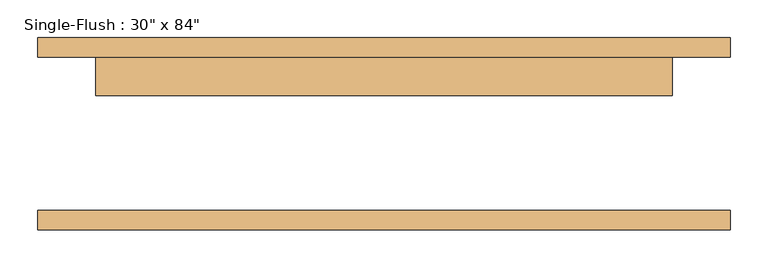
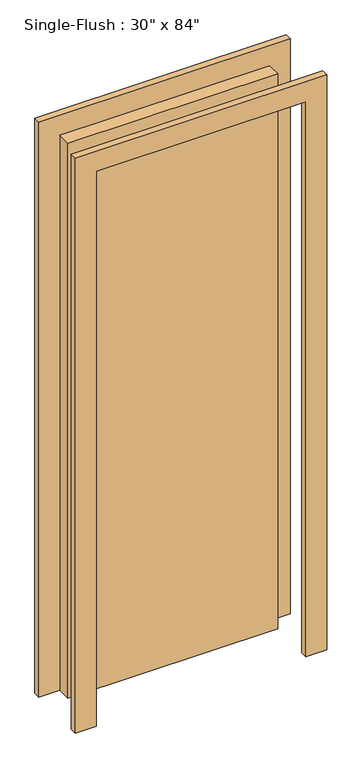
"""IFC4 building model written with IfcOpenShell, lengths in millimetres: door geometry."""

from ifc_helpers import new_model, si_unit, frame, origin, origin_with_axes, place, context, project, spatial, polyline, outline, extrude, source, transform, mapped, element, save


def door_b6acaa4e(model_context):
    return source(origin(), model_context, "Body", "SweptSolid", [
        extrude(outline(polyline([(2209.8, -457.2), (0.0, -457.2), (0.0, -381.0), (2133.6, -381.0), (2133.6, 381.0), (0.0, 381.0), (0.0, 457.2), (2209.8, 457.2), (2209.8, -457.2)])), frame((0.0, 101.6, 0.0), z_axis=(0.0, 1.0, 0.0), x_axis=(0.0, 0.0, 1.0)), (0.0, 0.0, 1.0), 25.4),
        extrude(outline(polyline([(2209.8, 457.2), (2209.8, -457.2), (0.0, -457.2), (0.0, -381.0), (2133.6, -381.0), (2133.6, 381.0), (0.0, 381.0), (0.0, 457.2), (2209.8, 457.2)])), frame((0.0, -127.0, 0.0), z_axis=(0.0, 1.0, 0.0), x_axis=(0.0, 0.0, 1.0)), (0.0, 0.0, 1.0), 25.4),
        extrude(outline(polyline([(381.0, 50.8), (-381.0, 50.8), (-381.0, 101.6), (381.0, 101.6), (381.0, 50.8)])), origin_with_axes(), (0.0, 0.0, 1.0), 2133.6),
    ])


if __name__ == "__main__":
    model = new_model("IFC4")
    model_context = context("Model", 3, world=origin())
    ifc_project = project(units=[si_unit("LENGTHUNIT", "METRE", prefix="MILLI")], contexts=[model_context])
    site = spatial("IfcSite", under=ifc_project)
    building = spatial("IfcBuilding", under=site)
    placement = place(None, origin())
    door_shape = door_b6acaa4e(model_context)
    element("IfcDoor", 1, ObjectType="Single-Flush : 30\" x 84\"", at=placement, inside=building, context=model_context, shape_type="MappedRepresentation", body=[
        mapped(door_shape, transform((0.0, 0.0, 0.0), x_axis=(1.0, 0.0, 0.0), y_axis=(0.0, 1.0, 0.0), z_axis=(0.0, 0.0, 1.0))),
    ])
    save(model, "model.ifc")

# Revit data of these elements
# Type "Single-Flush : 30\" x 84\""
#   Type Mark = "1"
#   Construction Type Id = "MDOOR"
#   Assembly Code = "C1020"
#   Analytic Construction = "Metal"
#   Thickness = 0' - 2"
#   Heat Transfer Coefficient (U) = 0.651978 BTU/(h·ft²·°F)
#   Height = 7' - 0"
#   Trim Projection Ext = 0' - 1"
#   Trim Projection Int = 0' - 1"
#   Trim Width = 0' - 3"
#   Width = 2' - 6"
#   Define Thermal Properties by = 1
#   Door Material = Door - Panel
#   Frame Material = Door - Frame
#   Visual Light Transmittance = 0
#   Solar Heat Gain Coefficient = 0
#   Function = (empty or 0)
#   Wall Closure = (empty or 0)
# Element 1 (IfcDoor, "Single-Flush : 30\" x 84\"")
#   Materials on its faces: "Door - Frame", "Door - Panel"
# Materials
#   "Door - Panel": class "Wood", colour RGB 210 159 95, transparency 0
#   "Door - Frame": colour RGB 118 70 51, transparency 0
